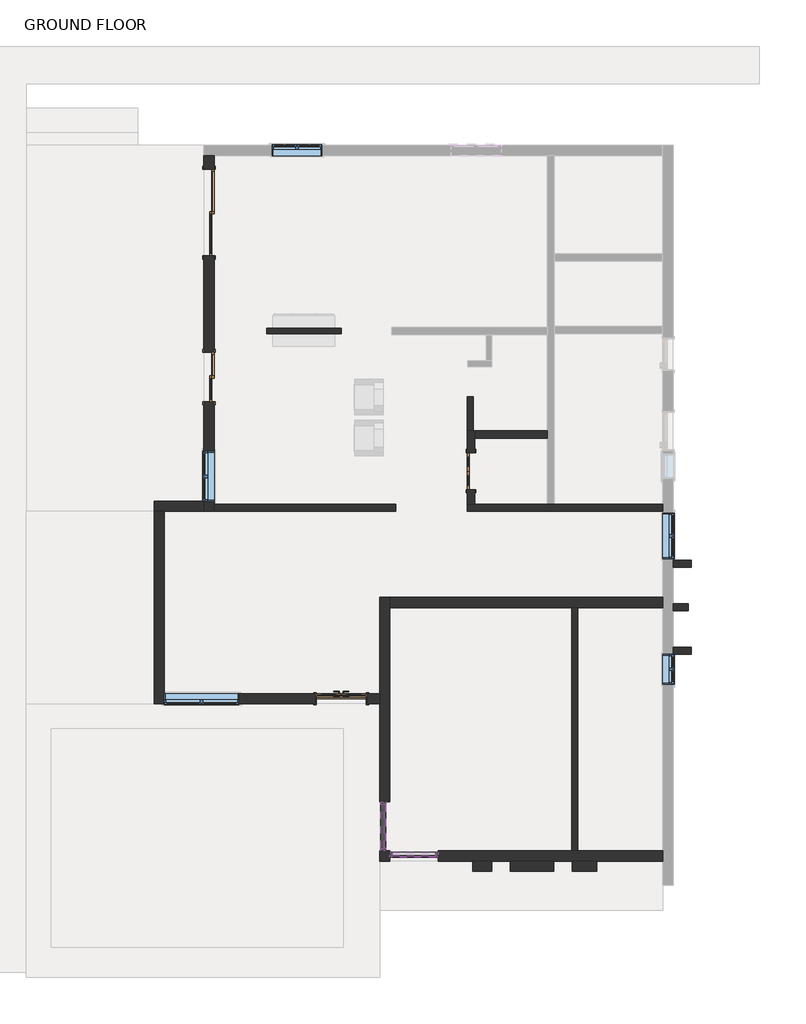
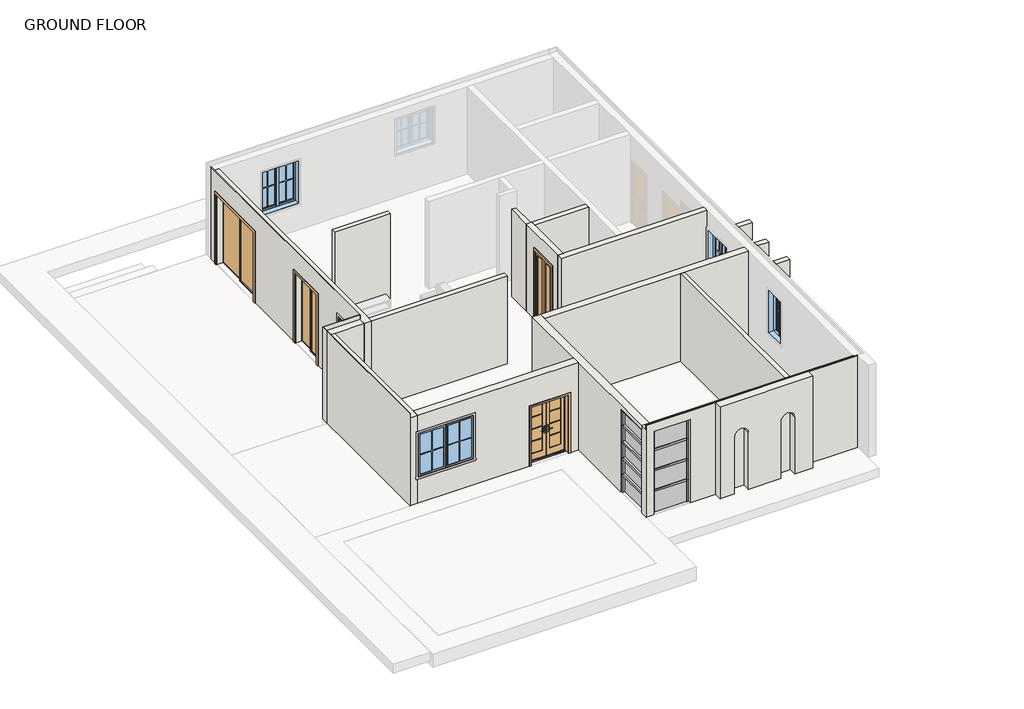
# One storey, part 1 of 2: 27 members, 18 walls, 9 plates, 5 windows, 4 doors.
"""IFC4 building model written with IfcOpenShell, lengths in millimetres."""

from ifc_helpers import new_model, si_unit, point, frame, frame_2d, origin, place, context, project, spatial, polyline, circle_curve, trimmed, segment, composite_curve, outline, extrude, faceted_brep, transform, mapped, element, save
from components import door_double_glass_3_725c6459, door_ed536266, door_double_sliding_6_53f3f6b1, door_ae07d0c6, member_2094b4cc, member_74e81316, member_bf0a6844, member_ab4f2237, member_d8a11517, member_bcb586ad, member_ae70dd35, member_aa870034, system_panel_glazed_a8ba4957, system_panel_glazed_1a26cfa3, system_panel_glazed_4987496d, system_panel_glazed_ecc42322, system_panel_glazed_0a58f99c, system_panel_glazed_1dd8fbf7, window_ba8015fa, window_casement_double_4_window_a93ed6b4, window_casement_double_4_9278a0c7, window_casement_double_6_75db422f

model = new_model("IFC4")

# Units and contexts
model_context = context("Model", 3, world=origin())
ifc_project = project(units=[si_unit("LENGTHUNIT", "METRE", prefix="MILLI")], contexts=[model_context])

# Site, building, storey
site = spatial("IfcSite", under=ifc_project)
building = spatial("IfcBuilding", under=site)
storey = spatial("IfcBuildingStorey", under=building, Name="GROUND FLOOR", Elevation=457.2)

# Doors
placement = place(None, origin())
door_double_glass_3_shape = door_double_glass_3_725c6459(model_context)
element("IfcDoor", 1, ObjectType="Door-Double-Glass : 3'", at=placement, inside=storey, context=model_context, shape_type="MappedRepresentation", body=[
    mapped(door_double_glass_3_shape, transform((1280.5251137, 1477.9935985, 457.2), x_axis=(0.0, 1.0, 0.0), y_axis=(-1.0, 0.0, 0.0), z_axis=(0.0, 0.0, 1.0))),
])
door_shape = door_ed536266(model_context)
element("IfcDoor", 2, ObjectType="Door-Double-Sliding : 48\" x 96\"", at=placement, inside=storey, context=model_context, shape_type="MappedRepresentation", body=[
    mapped(door_shape, transform((-5287.7561363, 3789.1221373, 457.2), x_axis=(0.0, -1.0, 0.0), y_axis=(1.0, 0.0, 0.0), z_axis=(0.0, 0.0, 1.0))),
])
door_double_sliding_6_shape = door_double_sliding_6_53f3f6b1(model_context)
element("IfcDoor", 3, ObjectType="Door-Double-Sliding : 6'", at=placement, inside=storey, context=model_context, shape_type="MappedRepresentation", body=[
    mapped(door_double_sliding_6_shape, transform((-5287.7561363, 7827.9935985, 457.2), x_axis=(0.0, -1.0, 0.0), y_axis=(1.0, 0.0, 0.0), z_axis=(0.0, 0.0, 1.0))),
])
door_2_shape = door_ae07d0c6(model_context)
element("IfcDoor", 4, ObjectType="Door-Exterior-Double-Full Glass-Wood_Clad : 48\" x 80\"", at=placement, inside=storey, context=model_context, shape_type="MappedRepresentation", body=[
    mapped(door_2_shape, transform((-1909.5561363, -4106.9516767, 457.2), x_axis=(1.0, 0.0, 0.0), y_axis=(0.0, 1.0, 0.0), z_axis=(0.0, 0.0, 1.0))),
])

# Members
member_shape = member_2094b4cc(model_context)
element("IfcMember", 5, ObjectType="Rectangular Mullion : 2.5\" x 5\" rectangular", at=placement, inside=storey, context=model_context, shape_type="MappedRepresentation", body=[
    mapped(member_shape, transform((-652.2561363, -7945.4064015, 3352.8), x_axis=(0.0, 0.0, 1.0), y_axis=(0.0, 1.0, 0.0), z_axis=(-1.0, 0.0, 0.0))),
])
member_2_shape = member_74e81316(model_context)
element("IfcMember", 6, ObjectType="Rectangular Mullion : 2.5\" x 5\" rectangular", at=placement, inside=storey, context=model_context, shape_type="MappedRepresentation", body=[
    mapped(member_2_shape, transform((-874.5061363, -7780.3064015, 3352.8), x_axis=(0.0, 0.0, 1.0), y_axis=(-1.0, 0.0, 0.0), z_axis=(0.0, -1.0, 0.0))),
])
member_3_shape = member_bf0a6844(model_context)
element("IfcMember", 7, ObjectType="Rectangular Mullion : 2.5\" x 5\" rectangular", at=placement, inside=storey, context=model_context, shape_type="MappedRepresentation", body=[
    mapped(member_3_shape, transform((-874.5061363, -7780.3064015, 2783.84), x_axis=(0.0, 0.0, 1.0), y_axis=(-1.0, 0.0, 0.0), z_axis=(0.0, -1.0, 0.0))),
])
element("IfcMember", 8, ObjectType="Rectangular Mullion : 2.5\" x 5\" rectangular", at=placement, inside=storey, context=model_context, shape_type="MappedRepresentation", body=[
    mapped(member_3_shape, transform((-874.5061363, -7780.3064015, 2214.88), x_axis=(0.0, 0.0, 1.0), y_axis=(-1.0, 0.0, 0.0), z_axis=(0.0, -1.0, 0.0))),
])
element("IfcMember", 9, ObjectType="Rectangular Mullion : 2.5\" x 5\" rectangular", at=placement, inside=storey, context=model_context, shape_type="MappedRepresentation", body=[
    mapped(member_3_shape, transform((-874.5061363, -7780.3064015, 1645.92), x_axis=(0.0, 0.0, 1.0), y_axis=(-1.0, 0.0, 0.0), z_axis=(0.0, -1.0, 0.0))),
])
element("IfcMember", 10, ObjectType="Rectangular Mullion : 2.5\" x 5\" rectangular", at=placement, inside=storey, context=model_context, shape_type="MappedRepresentation", body=[
    mapped(member_3_shape, transform((-874.5061363, -7780.3064015, 1076.96), x_axis=(0.0, 0.0, 1.0), y_axis=(-1.0, 0.0, 0.0), z_axis=(0.0, -1.0, 0.0))),
])
member_4_shape = member_ab4f2237(model_context)
element("IfcMember", 11, ObjectType="Rectangular Mullion : 2.5\" x 5\" rectangular", at=placement, inside=storey, context=model_context, shape_type="MappedRepresentation", body=[
    mapped(member_4_shape, transform((-874.5061363, -6637.3064015, 3352.8), x_axis=(0.0, 1.0, 0.0), y_axis=(-1.0, 0.0, 0.0), z_axis=(0.0, 0.0, 1.0))),
])
element("IfcMember", 12, ObjectType="Rectangular Mullion : 2.5\" x 5\" rectangular", at=placement, inside=storey, context=model_context, shape_type="MappedRepresentation", body=[
    mapped(member_4_shape, transform((-874.5061363, -7843.8064015, 2783.84), x_axis=(0.0, -1.0, 0.0), y_axis=(-1.0, 0.0, 0.0), z_axis=(0.0, 0.0, -1.0))),
])
element("IfcMember", 13, ObjectType="Rectangular Mullion : 2.5\" x 5\" rectangular", at=placement, inside=storey, context=model_context, shape_type="MappedRepresentation", body=[
    mapped(member_4_shape, transform((-874.5061363, -6637.3064015, 2783.84), x_axis=(0.0, 1.0, 0.0), y_axis=(-1.0, 0.0, 0.0), z_axis=(0.0, 0.0, 1.0))),
])
element("IfcMember", 14, ObjectType="Rectangular Mullion : 2.5\" x 5\" rectangular", at=placement, inside=storey, context=model_context, shape_type="MappedRepresentation", body=[
    mapped(member_4_shape, transform((-874.5061363, -6637.3064015, 2214.88), x_axis=(0.0, 1.0, 0.0), y_axis=(-1.0, 0.0, 0.0), z_axis=(0.0, 0.0, 1.0))),
])
element("IfcMember", 15, ObjectType="Rectangular Mullion : 2.5\" x 5\" rectangular", at=placement, inside=storey, context=model_context, shape_type="MappedRepresentation", body=[
    mapped(member_4_shape, transform((-874.5061363, -6637.3064015, 1645.92), x_axis=(0.0, 1.0, 0.0), y_axis=(-1.0, 0.0, 0.0), z_axis=(0.0, 0.0, 1.0))),
])
element("IfcMember", 16, ObjectType="Rectangular Mullion : 2.5\" x 5\" rectangular", at=placement, inside=storey, context=model_context, shape_type="MappedRepresentation", body=[
    mapped(member_4_shape, transform((-874.5061363, -7843.8064015, 2214.88), x_axis=(0.0, -1.0, 0.0), y_axis=(-1.0, 0.0, 0.0), z_axis=(0.0, 0.0, -1.0))),
])
element("IfcMember", 17, ObjectType="Rectangular Mullion : 2.5\" x 5\" rectangular", at=placement, inside=storey, context=model_context, shape_type="MappedRepresentation", body=[
    mapped(member_4_shape, transform((-874.5061363, -7843.8064015, 1645.92), x_axis=(0.0, -1.0, 0.0), y_axis=(-1.0, 0.0, 0.0), z_axis=(0.0, 0.0, -1.0))),
])
element("IfcMember", 18, ObjectType="Rectangular Mullion : 2.5\" x 5\" rectangular", at=placement, inside=storey, context=model_context, shape_type="MappedRepresentation", body=[
    mapped(member_4_shape, transform((-874.5061363, -7843.8064015, 1076.96), x_axis=(0.0, -1.0, 0.0), y_axis=(-1.0, 0.0, 0.0), z_axis=(0.0, 0.0, -1.0))),
])
member_5_shape = member_d8a11517(model_context)
element("IfcMember", 19, ObjectType="Rectangular Mullion : 2.5\" x 5\" rectangular", at=placement, inside=storey, context=model_context, shape_type="MappedRepresentation", body=[
    mapped(member_5_shape, transform((-874.5061363, -7843.8064015, 457.2), x_axis=(0.0, -1.0, 0.0), y_axis=(-1.0, 0.0, 0.0), z_axis=(0.0, 0.0, -1.0))),
])
element("IfcMember", 20, ObjectType="Rectangular Mullion : 2.5\" x 5\" rectangular", at=placement, inside=storey, context=model_context, shape_type="MappedRepresentation", body=[
    mapped(member_5_shape, transform((-874.5061363, -6637.3064015, 1076.96), x_axis=(0.0, 1.0, 0.0), y_axis=(-1.0, 0.0, 0.0), z_axis=(0.0, 0.0, 1.0))),
])
member_6_shape = member_bcb586ad(model_context)
element("IfcMember", 21, ObjectType="Rectangular Mullion : 2.5\" x 5\" rectangular", at=placement, inside=storey, context=model_context, shape_type="MappedRepresentation", body=[
    mapped(member_6_shape, transform((-652.2561363, -7945.4064015, 2641.6), x_axis=(0.0, 0.0, 1.0), y_axis=(0.0, 1.0, 0.0), z_axis=(-1.0, 0.0, 0.0))),
])
element("IfcMember", 22, ObjectType="Rectangular Mullion : 2.5\" x 5\" rectangular", at=placement, inside=storey, context=model_context, shape_type="MappedRepresentation", body=[
    mapped(member_6_shape, transform((-652.2561363, -7945.4064015, 1930.4), x_axis=(0.0, 0.0, 1.0), y_axis=(0.0, 1.0, 0.0), z_axis=(-1.0, 0.0, 0.0))),
])
element("IfcMember", 23, ObjectType="Rectangular Mullion : 2.5\" x 5\" rectangular", at=placement, inside=storey, context=model_context, shape_type="MappedRepresentation", body=[
    mapped(member_6_shape, transform((-652.2561363, -7945.4064015, 1219.2), x_axis=(0.0, 0.0, 1.0), y_axis=(0.0, 1.0, 0.0), z_axis=(-1.0, 0.0, 0.0))),
])
member_7_shape = member_ae70dd35(model_context)
element("IfcMember", 24, ObjectType="Rectangular Mullion : 2.5\" x 5\" rectangular", at=placement, inside=storey, context=model_context, shape_type="MappedRepresentation", body=[
    mapped(member_7_shape, transform((478.3084916, -7945.4064015, 3352.8), x_axis=(1.0, 0.0, 0.0), y_axis=(0.0, 1.0, 0.0), z_axis=(0.0, 0.0, 1.0))),
])
element("IfcMember", 25, ObjectType="Rectangular Mullion : 2.5\" x 5\" rectangular", at=placement, inside=storey, context=model_context, shape_type="MappedRepresentation", body=[
    mapped(member_7_shape, transform((-715.7561363, -7945.4064015, 2641.6), x_axis=(-1.0, 0.0, 0.0), y_axis=(0.0, 1.0, 0.0), z_axis=(0.0, 0.0, -1.0))),
])
element("IfcMember", 26, ObjectType="Rectangular Mullion : 2.5\" x 5\" rectangular", at=placement, inside=storey, context=model_context, shape_type="MappedRepresentation", body=[
    mapped(member_7_shape, transform((478.3084916, -7945.4064015, 2641.6), x_axis=(1.0, 0.0, 0.0), y_axis=(0.0, 1.0, 0.0), z_axis=(0.0, 0.0, 1.0))),
])
element("IfcMember", 27, ObjectType="Rectangular Mullion : 2.5\" x 5\" rectangular", at=placement, inside=storey, context=model_context, shape_type="MappedRepresentation", body=[
    mapped(member_7_shape, transform((478.3084916, -7945.4064015, 1930.4), x_axis=(1.0, 0.0, 0.0), y_axis=(0.0, 1.0, 0.0), z_axis=(0.0, 0.0, 1.0))),
])
element("IfcMember", 28, ObjectType="Rectangular Mullion : 2.5\" x 5\" rectangular", at=placement, inside=storey, context=model_context, shape_type="MappedRepresentation", body=[
    mapped(member_7_shape, transform((-715.7561363, -7945.4064015, 1930.4), x_axis=(-1.0, 0.0, 0.0), y_axis=(0.0, 1.0, 0.0), z_axis=(0.0, 0.0, -1.0))),
])
element("IfcMember", 29, ObjectType="Rectangular Mullion : 2.5\" x 5\" rectangular", at=placement, inside=storey, context=model_context, shape_type="MappedRepresentation", body=[
    mapped(member_7_shape, transform((-715.7561363, -7945.4064015, 1219.2), x_axis=(-1.0, 0.0, 0.0), y_axis=(0.0, 1.0, 0.0), z_axis=(0.0, 0.0, -1.0))),
])
member_8_shape = member_aa870034(model_context)
element("IfcMember", 30, ObjectType="Rectangular Mullion : 2.5\" x 5\" rectangular", at=placement, inside=storey, context=model_context, shape_type="MappedRepresentation", body=[
    mapped(member_8_shape, transform((-715.7561363, -7945.4064015, 457.2), x_axis=(-1.0, 0.0, 0.0), y_axis=(0.0, 1.0, 0.0), z_axis=(0.0, 0.0, -1.0))),
])
element("IfcMember", 31, ObjectType="Rectangular Mullion : 2.5\" x 5\" rectangular", at=placement, inside=storey, context=model_context, shape_type="MappedRepresentation", body=[
    mapped(member_8_shape, transform((478.3084916, -7945.4064015, 1219.2), x_axis=(1.0, 0.0, 0.0), y_axis=(0.0, 1.0, 0.0), z_axis=(0.0, 0.0, 1.0))),
])

# Plates
system_panel_glazed_shape = system_panel_glazed_a8ba4957(model_context)
element("IfcPlate", 32, ObjectType="System Panel : Glazed", at=placement, inside=storey, context=model_context, shape_type="MappedRepresentation", body=[
    mapped(system_panel_glazed_shape, transform((-874.5061363, -7240.5564015, 2815.59), x_axis=(0.0, -1.0, 0.0), y_axis=(1.0, 0.0, 0.0), z_axis=(0.0, 0.0, 1.0))),
])
system_panel_glazed_2_shape = system_panel_glazed_1a26cfa3(model_context)
element("IfcPlate", 33, ObjectType="System Panel : Glazed", at=placement, inside=storey, context=model_context, shape_type="MappedRepresentation", body=[
    mapped(system_panel_glazed_2_shape, transform((-874.5061363, -7240.5564015, 2246.63), x_axis=(0.0, -1.0, 0.0), y_axis=(1.0, 0.0, 0.0), z_axis=(0.0, 0.0, 1.0))),
])
element("IfcPlate", 34, ObjectType="System Panel : Glazed", at=placement, inside=storey, context=model_context, shape_type="MappedRepresentation", body=[
    mapped(system_panel_glazed_2_shape, transform((-874.5061363, -7240.5564015, 1677.67), x_axis=(0.0, -1.0, 0.0), y_axis=(1.0, 0.0, 0.0), z_axis=(0.0, 0.0, 1.0))),
])
element("IfcPlate", 35, ObjectType="System Panel : Glazed", at=placement, inside=storey, context=model_context, shape_type="MappedRepresentation", body=[
    mapped(system_panel_glazed_2_shape, transform((-874.5061363, -7240.5564015, 1108.71), x_axis=(0.0, -1.0, 0.0), y_axis=(1.0, 0.0, 0.0), z_axis=(0.0, 0.0, 1.0))),
])
system_panel_glazed_3_shape = system_panel_glazed_4987496d(model_context)
element("IfcPlate", 36, ObjectType="System Panel : Glazed", at=placement, inside=storey, context=model_context, shape_type="MappedRepresentation", body=[
    mapped(system_panel_glazed_3_shape, transform((-874.5061363, -7240.5564015, 457.2), x_axis=(0.0, -1.0, 0.0), y_axis=(1.0, 0.0, 0.0), z_axis=(0.0, 0.0, 1.0))),
])
system_panel_glazed_4_shape = system_panel_glazed_ecc42322(model_context)
element("IfcPlate", 37, ObjectType="System Panel : Glazed", at=placement, inside=storey, context=model_context, shape_type="MappedRepresentation", body=[
    mapped(system_panel_glazed_4_shape, transform((-118.7238223, -7945.4064015, 2673.35), x_axis=(-1.0, 0.0, 0.0), y_axis=(0.0, -1.0, 0.0), z_axis=(0.0, 0.0, 1.0))),
])
system_panel_glazed_5_shape = system_panel_glazed_0a58f99c(model_context)
element("IfcPlate", 38, ObjectType="System Panel : Glazed", at=placement, inside=storey, context=model_context, shape_type="MappedRepresentation", body=[
    mapped(system_panel_glazed_5_shape, transform((-118.7238223, -7945.4064015, 1962.15), x_axis=(-1.0, 0.0, 0.0), y_axis=(0.0, -1.0, 0.0), z_axis=(0.0, 0.0, 1.0))),
])
element("IfcPlate", 39, ObjectType="System Panel : Glazed", at=placement, inside=storey, context=model_context, shape_type="MappedRepresentation", body=[
    mapped(system_panel_glazed_5_shape, transform((-118.7238223, -7945.4064015, 1250.95), x_axis=(-1.0, 0.0, 0.0), y_axis=(0.0, -1.0, 0.0), z_axis=(0.0, 0.0, 1.0))),
])
system_panel_glazed_6_shape = system_panel_glazed_1dd8fbf7(model_context)
element("IfcPlate", 40, ObjectType="System Panel : Glazed", at=placement, inside=storey, context=model_context, shape_type="MappedRepresentation", body=[
    mapped(system_panel_glazed_6_shape, transform((-118.7238223, -7945.4064015, 457.2), x_axis=(-1.0, 0.0, 0.0), y_axis=(0.0, -1.0, 0.0), z_axis=(0.0, 0.0, 1.0))),
])

# Walls
element("IfcWall", 41, ObjectType="4.5\"", at=placement, inside=storey, context=model_context, shape_type="SweptSolid", body=[
    extrude(outline(polyline([(3754.6438637, -7843.8064015), (3754.6438637, -1874.8064015), (3894.3438637, -1874.8064015), (3894.3438637, -7843.8064015), (3754.6438637, -7843.8064015)])), frame((0.0, 0.0, 457.2), z_axis=(0.0, 0.0, 1.0), x_axis=(1.0, 0.0, 0.0)), (0.0, 0.0, 1.0), 3048.0),
])
element("IfcWall", 42, ObjectType="4.5\"", at=placement, inside=storey, context=model_context, shape_type="SweptSolid", body=[
    extrude(outline(polyline([(1328.9438637, 3306.7935985), (1328.9438637, 2468.5935985), (1189.2438637, 2468.5935985), (1189.2438637, 3306.7935985), (1328.9438637, 3306.7935985)])), frame((0.0, 0.0, 457.2), z_axis=(0.0, 0.0, 1.0), x_axis=(1.0, 0.0, 0.0)), (0.0, 0.0, 1.0), 3048.0),
])
element("IfcWall", 43, ObjectType="4.5\"", at=placement, inside=storey, context=model_context, shape_type="SweptSolid", body=[
    extrude(outline(polyline([(-3743.6809093, 4989.3322749), (-1914.8809093, 4989.3322749), (-1914.8809093, 4849.6322749), (-3743.6809093, 4849.6322749), (-3743.6809093, 4989.3322749)])), frame((0.0, 0.0, 457.2), z_axis=(0.0, 0.0, 1.0), x_axis=(1.0, 0.0, 0.0)), (0.0, 0.0, 1.0), 3048.0),
])
element("IfcWall", 44, ObjectType="6\" WALL", at=placement, inside=storey, context=model_context, shape_type="Brep", body=[
    faceted_brep([(5990.1084916, 665.1935985, 457.2), (3322.8438637, 665.1935985, 457.2), (3145.0438637, 665.1935985, 457.2), (1367.0438637, 665.1935985, 457.2), (1189.2438637, 665.1935985, 457.2), (1189.2438637, 665.1935985, 3505.2), (5990.1084916, 665.1935985, 3505.2), (1189.2438637, 487.3935985, 457.2), (5990.1084916, 487.3935985, 457.2), (5990.1084916, 487.3935985, 3505.2), (1189.2438637, 487.3935985, 3505.2)], [[[0, 1, 2, 3, 4, 5, 6]], [[7, 8, 9, 10]], [[4, 3, 2, 1, 0, 8, 7]], [[8, 0, 6, 9]], [[4, 7, 10, 5]], [[6, 5, 10, 9]]]),
])
element("IfcWall", 45, ObjectType="6\" WALL", at=placement, inside=storey, context=model_context, shape_type="Brep", body=[
    faceted_brep([(1367.0438637, 1935.1935985, 2895.6), (1367.0438637, 1935.1935985, 457.2), (1367.0438637, 2290.7935985, 457.2), (1367.0438637, 2468.5935985, 457.2), (1367.0438637, 2468.5935985, 3505.2), (1367.0438637, 665.1935985, 3505.2), (1367.0438637, 665.1935985, 457.2), (1367.0438637, 1020.7935985, 457.2), (1367.0438637, 1020.7935985, 2895.6), (1189.2438637, 1935.1935985, 457.2), (1189.2438637, 1935.1935985, 2895.6), (1189.2438637, 1020.7935985, 2895.6), (1189.2438637, 1020.7935985, 457.2), (1189.2438637, 665.1935985, 457.2), (1189.2438637, 665.1935985, 3505.2), (1189.2438637, 2468.5935985, 3505.2), (1189.2438637, 2468.5935985, 457.2), (1328.9438637, 2468.5935985, 457.2)], [[[0, 1, 2, 3, 4, 5, 6, 7, 8]], [[9, 10, 11, 12, 13, 14, 15, 16]], [[6, 13, 12, 7]], [[16, 17, 3, 2, 1, 9]], [[13, 6, 5, 14]], [[3, 17, 16, 15, 4]], [[10, 9, 1, 0]], [[11, 10, 0, 8]], [[12, 11, 8, 7]], [[5, 4, 15, 14]]]),
])
element("IfcWall", 46, ObjectType="6\" WALL", at=placement, inside=storey, context=model_context, shape_type="SweptSolid", body=[
    extrude(outline(polyline([(3145.0438637, 2290.7935985), (1367.0438637, 2290.7935985), (1367.0438637, 2468.5935985), (3145.0438637, 2468.5935985), (3145.0438637, 2290.7935985)])), frame((0.0, 0.0, 457.2), z_axis=(0.0, 0.0, 1.0), x_axis=(1.0, 0.0, 0.0)), (0.0, 0.0, 1.0), 3048.0),
])
element("IfcWall", 47, ObjectType="6\" WALL", at=placement, inside=storey, context=model_context, shape_type="SweptSolid", body=[
    extrude(outline(polyline([(-5033.7561363, 664.9221371), (-576.2004467, 664.9221371), (-576.2004467, 487.1221371), (-5033.7561363, 487.1221371), (-5033.7561363, 664.9221371)])), frame((0.0, 0.0, 457.2), z_axis=(0.0, 0.0, 1.0), x_axis=(1.0, 0.0, 0.0)), (0.0, 0.0, 1.0), 3048.0),
])
element("IfcWall", 48, ObjectType="6\" WALL", at=placement, inside=storey, context=model_context, shape_type="SweptSolid", body=[
    extrude(outline(polyline([(6688.3438637, -885.2318739), (6244.1084916, -885.2318739), (6244.1084916, -707.4318739), (6688.3438637, -707.4318739), (6688.3438637, -885.2318739)])), frame((0.0, 0.0, 457.2), z_axis=(0.0, 0.0, 1.0), x_axis=(1.0, 0.0, 0.0)), (0.0, 0.0, 1.0), 3200.4),
])
element("IfcWall", 49, ObjectType="6\" WALL", at=placement, inside=storey, context=model_context, shape_type="SweptSolid", body=[
    extrude(outline(polyline([(6244.1084916, -2840.9358398), (6688.3438637, -2840.9358398), (6688.3438637, -3018.7358398), (6244.1084916, -3018.7358398), (6244.1084916, -2840.9358398)])), frame((0.0, 0.0, 457.2), z_axis=(0.0, 0.0, 1.0), x_axis=(1.0, 0.0, 0.0)), (0.0, 0.0, 1.0), 3200.4),
])
element("IfcWall", 50, ObjectType="6\" WALL", at=placement, inside=storey, context=model_context, shape_type="SweptSolid", body=[
    extrude(outline(polyline([(6244.1084916, -1774.2318739), (6612.1438637, -1774.2318739), (6612.1438637, -1952.0318739), (6244.1084916, -1952.0318739), (6244.1084916, -1774.2318739)])), frame((0.0, 0.0, 457.2), z_axis=(0.0, 0.0, 1.0), x_axis=(1.0, 0.0, 0.0)), (0.0, 0.0, 1.0), 3200.4),
])
element("IfcWall", 51, ObjectType="9\"", at=placement, inside=storey, context=model_context, shape_type="Brep", body=[
    faceted_brep([(5990.1084916, -8097.8064015, 3657.6), (-969.7561363, -8097.8064015, 3657.6), (-969.7561363, -8097.8064015, 457.2), (-715.7561363, -8097.8064015, 457.2), (-715.7561363, -8097.8064015, 3352.8), (478.3084916, -8097.8064015, 3352.8), (478.3084916, -8097.8064015, 457.2), (5990.1084916, -8097.8064015, 457.2), (5990.1084916, -7843.8064015, 457.2), (3894.3438637, -7843.8064015, 457.2), (3754.6438637, -7843.8064015, 457.2), (478.3084916, -7843.8064015, 457.2), (478.3084916, -7843.8064015, 3352.8), (-715.7561363, -7843.8064015, 3352.8), (-715.7561363, -7843.8064015, 457.2), (-969.7561363, -7843.8064015, 457.2), (-969.7561363, -7843.8064015, 3352.8), (-969.7561363, -7843.8064015, 3505.2), (-715.7561363, -7843.8064015, 3505.2), (3754.6438637, -7843.8064015, 3505.2), (3894.3438637, -7843.8064015, 3505.2), (5990.1084916, -7843.8064015, 3505.2), (5990.1084916, -8085.1064015, 3657.6), (-969.7561363, -8085.1064015, 3657.6), (5990.1084916, -8085.1064015, 3505.2), (-969.7561363, -8085.1064015, 3505.2)], [[[0, 1, 2, 3, 4, 5, 6, 7]], [[8, 9, 10, 11, 12, 13, 14, 15, 16, 17, 18, 19, 20, 21]], [[8, 7, 6, 11, 10, 9]], [[3, 2, 15, 14]], [[1, 0, 22, 23]], [[0, 7, 8, 21, 24, 22]], [[5, 12, 11, 6]], [[12, 5, 4, 13]], [[13, 4, 3, 14]], [[2, 1, 23, 25, 17, 16, 15]], [[25, 24, 21, 20, 19, 18, 17]], [[24, 25, 23, 22]]]),
])
element("IfcWall", 52, ObjectType="9\"", at=placement, inside=storey, context=model_context, shape_type="Brep", body=[
    faceted_brep([(-5287.7561363, 9224.9935985, 3657.6), (-5287.7561363, 9224.9935985, 457.2), (-5287.7561363, 8894.7935985, 457.2), (-5287.7561363, 8894.7935985, 2895.6), (-5287.7561363, 6761.1935985, 2895.6), (-5287.7561363, 6761.1935985, 457.2), (-5287.7561363, 4398.7221373, 457.2), (-5287.7561363, 4398.7221373, 2895.6), (-5287.7561363, 3179.5221373, 2895.6), (-5287.7561363, 3179.5221373, 457.2), (-5287.7561363, 741.1221373, 457.2), (-5287.7561363, 487.1221373, 457.2), (-5287.7561363, 487.1221373, 3505.2), (-5287.7561363, 728.4221373, 3505.2), (-5287.7561363, 728.4221373, 3657.6), (-5287.7561363, 741.1221373, 3657.6), (-5287.7561363, 1960.3221373, 1371.6), (-5287.7561363, 1960.3221373, 2895.6), (-5287.7561363, 741.1221373, 2895.6), (-5287.7561363, 741.1221373, 1371.6), (-5033.7561363, 4398.7221373, 2895.6), (-5033.7561363, 4398.7221373, 457.2), (-5033.7561363, 6761.1935985, 457.2), (-5033.7561363, 6761.1935985, 2895.6), (-5033.7561363, 8894.7935985, 2895.6), (-5033.7561363, 8894.7935985, 457.2), (-5033.7561363, 9224.9935985, 457.2), (-5033.7561363, 9224.9935985, 3505.2), (-5033.7561363, 664.9221371, 3505.2), (-5033.7561363, 487.1221373, 3505.2), (-5033.7561363, 487.1221373, 457.2), (-5033.7561363, 664.9221371, 457.2), (-5033.7561363, 3179.5221373, 457.2), (-5033.7561363, 3179.5221373, 2895.6), (-5033.7561363, 1960.3221373, 2895.6), (-5033.7561363, 1960.3221373, 1371.6), (-5033.7561363, 741.1221373, 1371.6), (-5033.7561363, 741.1221373, 2895.6), (-5275.0561363, 728.4221373, 3657.6), (-5275.0561363, 9224.9935985, 3657.6), (-5275.0561363, 9224.9935985, 3505.2), (-5275.0561363, 728.4221373, 3505.2)], [[[0, 1, 2, 3, 4, 5, 6, 7, 8, 9, 10, 11, 12, 13, 14, 15], [16, 17, 18, 19]], [[20, 21, 22, 23, 24, 25, 26, 27, 28, 29, 30, 31, 32, 33], [34, 35, 36, 37]], [[1, 26, 25, 2]], [[30, 11, 10, 9, 32, 31]], [[21, 6, 5, 22]], [[0, 15, 14, 38, 39]], [[1, 0, 39, 40, 27, 26]], [[11, 30, 29, 12]], [[35, 34, 17, 16]], [[36, 35, 16, 19]], [[37, 36, 19, 18]], [[34, 37, 18, 17]], [[21, 20, 7, 6]], [[33, 32, 9, 8]], [[20, 33, 8, 7]], [[25, 24, 3, 2]], [[23, 22, 5, 4]], [[24, 23, 4, 3]], [[40, 41, 13, 12, 29, 28, 27]], [[41, 38, 14, 13]], [[38, 41, 40, 39]]]),
])
element("IfcWall", 53, ObjectType="9\"", at=placement, inside=storey, context=model_context, shape_type="Brep", body=[
    faceted_brep([(-5287.7561363, 741.1221373, 457.2), (-6507.1004467, 741.1221373, 457.2), (-6507.1004467, 741.1221373, 3657.6), (-5287.7561363, 741.1221373, 3657.6), (-5287.7561363, 741.1221373, 2895.6), (-5287.7561363, 741.1221373, 1371.6), (-6507.1004467, 487.1221373, 457.2), (-6253.1004467, 487.1221373, 457.2), (-5287.7561363, 487.1221373, 457.2), (-5287.7561363, 487.1221373, 3505.2), (-6253.1004467, 487.1221373, 3505.2), (-6494.4004467, 487.1221373, 3505.2), (-6494.4004467, 487.1221373, 3657.6), (-6507.1004467, 487.1221373, 3657.6), (-6494.4004467, 728.4221373, 3657.6), (-5287.7561363, 728.4221373, 3657.6), (-5287.7561363, 728.4221373, 3505.2), (-6494.4004467, 728.4221373, 3505.2)], [[[0, 1, 2, 3, 4, 5]], [[6, 7, 8, 9, 10, 11, 12, 13]], [[1, 0, 8, 7, 6]], [[3, 2, 13, 12, 14, 15]], [[0, 5, 4, 3, 15, 16, 9, 8]], [[2, 1, 6, 13]], [[16, 17, 11, 10, 9]], [[17, 14, 12, 11]], [[14, 17, 16, 15]]]),
])
element("IfcWall", 54, ObjectType="9\"", at=placement, inside=storey, context=model_context, shape_type="Brep", body=[
    faceted_brep([(-6507.1004467, 487.1221373, 457.2), (-6507.1004467, -4237.1266767, 457.2), (-6507.1004467, -4237.1266767, 3657.6), (-6507.1004467, 487.1221373, 3657.6), (-6253.1004467, -4237.1266767, 457.2), (-6253.1004467, -3983.1266767, 457.2), (-6253.1004467, 487.1221373, 457.2), (-6253.1004467, 487.1221373, 3505.2), (-6253.1004467, -3983.1266767, 3505.2), (-6253.1004467, -4237.1266767, 3505.2), (-6253.1004467, -4237.1266767, 2895.6), (-6253.1004467, -4237.1266767, 1371.6), (-6494.4004467, -4237.1266767, 3657.6), (-6494.4004467, 487.1221373, 3657.6), (-6494.4004467, 487.1221373, 3505.2), (-6494.4004467, -4237.1266767, 3505.2)], [[[0, 1, 2, 3]], [[4, 5, 6, 7, 8, 9, 10, 11]], [[1, 0, 6, 5, 4]], [[3, 2, 12, 13]], [[0, 3, 13, 14, 7, 6]], [[2, 1, 4, 11, 10, 9, 15, 12]], [[14, 15, 9, 8, 7]], [[15, 14, 13, 12]]]),
])
element("IfcWall", 55, ObjectType="9\"", at=placement, inside=storey, context=model_context, shape_type="SweptSolid", body=[
    extrude(outline(polyline([(1371.6, -4424.3004467), (1371.6, -6253.1004467), (457.2, -6253.1004467), (457.2, -2544.5561363), (2514.6, -2544.5561363), (2514.6, -1274.5561363), (457.2, -1274.5561363), (457.2, -969.7561363), (3505.2, -969.7561363), (3505.2, -6253.1004467), (2895.6, -6253.1004467), (2895.6, -4424.3004467), (1371.6, -4424.3004467)])), frame((0.0, -4237.1266767, 0.0), z_axis=(0.0, 1.0, 0.0), x_axis=(0.0, 0.0, 1.0)), (0.0, 0.0, 1.0), 254.0),
])
element("IfcWall", 56, ObjectType="9\"", at=placement, inside=storey, context=model_context, shape_type="Brep", body=[
    faceted_brep([(-715.7561363, -6637.3064015, 457.2), (-715.7561363, -1874.8064015, 457.2), (-715.7561363, -1620.8064015, 457.2), (-715.7561363, -1620.8064015, 3505.2), (-715.7561363, -7843.8064015, 3505.2), (-715.7561363, -7843.8064015, 3352.8), (-715.7561363, -6637.3064015, 3352.8), (-969.7561363, -1620.8064015, 457.2), (-969.7561363, -3983.1266767, 457.2), (-969.7561363, -4237.1266767, 457.2), (-969.7561363, -6637.3064015, 457.2), (-969.7561363, -6637.3064015, 3352.8), (-969.7561363, -7843.8064015, 3352.8), (-969.7561363, -7843.8064015, 3505.2), (-969.7561363, -4237.1266767, 3505.2), (-969.7561363, -3983.1266767, 3505.2), (-969.7561363, -1620.8064015, 3505.2)], [[[0, 1, 2, 3, 4, 5, 6]], [[7, 8, 9, 10, 11, 12, 13, 14, 15, 16]], [[7, 2, 1, 0, 10, 9, 8]], [[2, 7, 16, 3]], [[12, 5, 4, 13]], [[6, 11, 10, 0]], [[11, 6, 5, 12]], [[4, 3, 16, 15, 14, 13]]]),
])
element("IfcWall", 57, ObjectType="9\"", at=placement, inside=storey, context=model_context, shape_type="Brep", body=[
    faceted_brep([(-715.7561363, -1874.8064015, 457.2), (3754.6438637, -1874.8064015, 457.2), (3894.3438637, -1874.8064015, 457.2), (5990.1084916, -1874.8064015, 457.2), (5990.1084916, -1874.8064015, 3505.2), (-715.7561363, -1874.8064015, 3505.2), (5990.1084916, -1620.8064015, 457.2), (-715.7561363, -1620.8064015, 457.2), (-715.7561363, -1620.8064015, 3505.2), (5990.1084916, -1620.8064015, 3505.2)], [[[0, 1, 2, 3, 4, 5]], [[6, 7, 8, 9]], [[3, 2, 1, 0, 7, 6]], [[7, 0, 5, 8]], [[3, 6, 9, 4]], [[5, 4, 9, 8]]]),
])
element("IfcWall", 58, ObjectType="9\"", at=placement, inside=storey, context=model_context, shape_type="SweptSolid", body=[
    extrude(outline(composite_curve([segment(polyline([(457.2, 1315.4507424), (457.2, 1786.1438637), (2438.4, 1786.1438637)]), True, "CONTINUOUS"), segment(trimmed(circle_curve(frame_2d((2438.4, 2014.7438637)), 228.6), [point((2438.4, 1786.1438637))], [point((2438.4, 2243.3438637))], True, "CARTESIAN"), True, "CONTINUOUS"), segment(polyline([(2438.4, 2243.3438637), (457.2, 2243.3438637), (457.2, 3310.1438637), (2438.4, 3310.1438637)]), True, "CONTINUOUS"), segment(trimmed(circle_curve(frame_2d((2438.4, 3538.7438637)), 228.6), [point((2438.4, 3310.1438637))], [point((2438.4, 3767.3438637))], True, "CARTESIAN"), True, "CONTINUOUS"), segment(polyline([(2438.4, 3767.3438637), (457.2, 3767.3438637), (457.2, 4363.4507424), (3657.6, 4363.4507424), (3657.6, 1315.4507424), (457.2, 1315.4507424)]), True, "CONTINUOUS")], self_intersect=False)), frame((0.0, -8351.8064015, 0.0), z_axis=(0.0, 1.0, 0.0), x_axis=(0.0, 0.0, 1.0)), (0.0, 0.0, 1.0), 254.0),
])

# Windows
window_shape = window_ba8015fa(model_context)
element("IfcWindow", 59, ObjectType="Window-Casement-Double : 2'5\"", at=placement, inside=storey, context=model_context, shape_type="MappedRepresentation", body=[
    mapped(window_shape, transform((6117.1084916, -3387.0358398, 457.2), x_axis=(0.0, -1.0, 0.0), y_axis=(1.0, 0.0, 0.0), z_axis=(0.0, 0.0, 1.0))),
])
window_casement_double_4_window_shape = window_casement_double_4_window_a93ed6b4(model_context)
element("IfcWindow", 60, ObjectType="Window-Casement-Double : 4 window", at=placement, inside=storey, context=model_context, shape_type="MappedRepresentation", body=[
    mapped(window_casement_double_4_window_shape, transform((-5160.7561363, 1350.7221373, 457.2), x_axis=(0.0, 1.0, 0.0), y_axis=(-1.0, 0.0, 0.0), z_axis=(0.0, 0.0, 1.0))),
])
element("IfcWindow", 61, ObjectType="Window-Casement-Double : 4 window", at=placement, inside=storey, context=model_context, shape_type="MappedRepresentation", body=[
    mapped(window_casement_double_4_window_shape, transform((-2996.5357334, 9351.9935985, 457.2), x_axis=(1.0, 0.0, 0.0), y_axis=(0.0, 1.0, 0.0), z_axis=(0.0, 0.0, 1.0))),
])
window_casement_double_4_shape = window_casement_double_4_9278a0c7(model_context)
element("IfcWindow", 62, ObjectType="Window-Casement-Double : 4'", at=placement, inside=storey, context=model_context, shape_type="MappedRepresentation", body=[
    mapped(window_casement_double_4_shape, transform((6117.1084916, -110.0191377, 457.2), x_axis=(0.0, -1.0, 0.0), y_axis=(1.0, 0.0, 0.0), z_axis=(0.0, 0.0, 1.0))),
])
window_casement_double_6_shape = window_casement_double_6_75db422f(model_context)
element("IfcWindow", 63, ObjectType="Window-Casement-Double : 6'", at=placement, inside=storey, context=model_context, shape_type="MappedRepresentation", body=[
    mapped(window_casement_double_6_shape, transform((-5338.7004467, -4110.1266767, 457.2), x_axis=(-1.0, 0.0, 0.0), y_axis=(0.0, -1.0, 0.0), z_axis=(0.0, 0.0, 1.0))),
])

save(model, "model.ifc")

# Revit data of these elements
# Type "Door-Double-Glass : 3'"
#   Type Mark = "14"
#   Construction Type Id = "opn-d45"
#   Assembly Code = "C1020"
#   Analytic Construction = "Wood frame, double glass door "
#   W = 1' - 6"
#   Thickness = 0' - 2"
#   Thermal Resistance (R) = 1.8150 (h·ft²·°F)/BTU
#   Swing Angle [instance default] = 90.00°
#   Heat Transfer Coefficient (U) = 0.5510 BTU/(h·ft²·°F)
#   Height = 8' - 0"
#   Bottom Rail = 0' - 4"
#   Top Rail = 0' - 4"
#   Stiles = 0' - 4"
#   Trim Projection = 0' - 1"
#   Trim Width = 0' - 3"
#   Width = 3' - 0"
#   Define Thermal Properties by = 1
#   Glazing = Glass
#   Panel Material = Wood - Birch - Solid Stained Light Low Gloss
#   Trim Material = Paint - Sienna
#   Visual Light Transmittance = 0
#   Solar Heat Gain Coefficient = 0
#   Function = (empty or 0)
#   Wall Closure = (empty or 0)
# Type "Door-Double-Sliding : 48\" x 96\""
#   Type Mark = "8"
#   Construction Type Id = "opn-d45"
#   Assembly Code = "C1020"
#   Analytic Construction = "Wood frame, double glass door "
#   Thickness = 0' - 2"
#   Thermal Resistance (R) = 1.8150 (h·ft²·°F)/BTU
#   Heat Transfer Coefficient (U) = 0.5510 BTU/(h·ft²·°F)
#   Height = 8' - 0"
#   Rail Width = 0' - 2"
#   Stiles = 0' - 2"
#   Trim Projection Ext = 0' - 1"
#   Trim Projection Int = 0' - 1"
#   Trim Width = 0' - 3"
#   Width = 4' - 0"
#   Define Thermal Properties by = 1
#   Glazing = Glass
#   Panel Material = Wood - Birch - Solid Stained Light Low Gloss
#   Trim Material = Paint - Sienna
#   Visual Light Transmittance = 0
#   Solar Heat Gain Coefficient = 0
#   Function = (empty or 0)
#   Wall Closure = (empty or 0)
# Type "Door-Double-Sliding : 6'"
#   Type Mark = "9"
#   Construction Type Id = "opn-d45"
#   Assembly Code = "C1020"
#   Analytic Construction = "Wood frame, double glass door "
#   Thickness = 0' - 2"
#   Thermal Resistance (R) = 1.8150 (h·ft²·°F)/BTU
#   Heat Transfer Coefficient (U) = 0.5510 BTU/(h·ft²·°F)
#   Height = 8' - 0"
#   Rail Width = 0' - 2"
#   Stiles = 0' - 2"
#   Trim Projection Ext = 0' - 1"
#   Trim Projection Int = 0' - 1"
#   Trim Width = 0' - 3"
#   Width = 7' - 0"
#   Define Thermal Properties by = 1
#   Glazing = Glass
#   Panel Material = Wood - Birch - Solid Stained Light Low Gloss
#   Trim Material = Paint - Sienna
#   Visual Light Transmittance = 0
#   Solar Heat Gain Coefficient = 0
#   Function = (empty or 0)
#   Wall Closure = (empty or 0)
# Type "Door-Exterior-Double-Full Glass-Wood_Clad : 48\" x 80\""
#   Type Mark = "16"
#   Assembly Code = "B2030100"
#   Analytic Construction = "French door, wood frame with double glass"
#   Top Rail = 0' - 4 11/16"
#   Threshold Offset [instance default] = 0' - 0 1/2"
#   Thickness = 0' - 1 3/8"
#   Thermal Resistance (R) = 1.9158 (h·ft²·°F)/BTU
#   Swing Angle [instance default] = 90.00°
#   Stiles = 0' - 4 3/4"
#   Rough Width = 4' - 2"
#   Rough Height = 6' - 9"
#   Panel Width = 2' - 0"
#   Door Offset [instance default] = 0' - 0"
#   Height = 6' - 8"
#   Width = 4' - 0"
#   Heat Transfer Coefficient (U) = 0.5220 BTU/(h·ft²·°F)
#   Bottom Rail = 0' - 9 1/8"
#   Exterior Trim [instance default] = yes
#   Threshold [instance default] = yes
#   Show Grill [instance default] = yes
#   Function = 1
#   Trim Material = Cherry
#   Threshold Material = Cherry
#   Panel Material = Cherry
#   Glazing = Glass
#   Frame Material = Cherry
#   Door Handle Material = Aluminum
#   Visual Light Transmittance = 0
#   Solar Heat Gain Coefficient = 0
#   Wall Closure = (empty or 0)
#   Construction Type = (empty or 0)
# Type "Rectangular Mullion : 2.5\" x 5\" rectangular"
#   built-in parameter 1007304 = 0.416667 (stored number, unit not read)
#   built-in parameter 1007301 = 0.104167 (stored number, unit not read)
#   built-in parameter 1007300 = 0.104167 (stored number, unit not read)
# Type "System Panel : Glazed"
#   Construction Type Id = "GSP4R"
#   Analytic Construction = "1/8 in Pilkington single glazing"
#   Visual Light Transmittance = 0.9
#   Solar Heat Gain Coefficient = 0.86
#   Heat Transfer Coefficient (U) = 1.18115 BTU/(h·ft²·°F)
#   Define Thermal Properties by = 1
# Type "4.5\""
#   Assembly Code = "B2010"
#   Layers, outside or top first: 0' - 0 1/2" no material (function 4); 0' - 4 1/2" "Acoustic Ceiling Tile 24 x 24" (function 1); 0' - 0 1/2" no material (function 4)
# Type "6\" WALL"
#   Assembly Code = "B2010"
#   Layers, outside or top first: 0' - 0 1/2" no material (function 4); 0' - 6" no material (function 1); 0' - 0 1/2" no material (function 4)
# Type "9\""
#   Assembly Code = "B2010"
#   Layers, outside or top first: 0' - 0 1/2" no material (function 4); 0' - 9" no material (function 1); 0' - 0 1/2" no material (function 4)
# Type "Window-Casement-Double : 2'5\""
#   Type Mark = "19"
#   Fire Rating = "0.5h"
#   Assembly Code = "B2020100"
#   Analytic Construction = "Double glazing - domestic"
#   Frame Extension [instance default] = 0' - 0 1/4"
#   Window Inset [instance default] = 0' - 0"
#   Wall Thickness [instance default] = 0' - 6"
#   Interior Wall Closure [instance default] = 0' - 2 1/4"
#   Half Width = 1' - 2 1/2"
#   Visual Light Transmittance = 0.81
#   Thermal Resistance (R) = 1.8146 (h·ft²·°F)/BTU
#   Solar Heat Gain Coefficient = 0.76
#   Rough Width = 2' - 5 1/2"
#   Rough Height = 5' - 0 1/2"
#   Height = 5' - 0"
#   Heat Transfer Coefficient (U) = 0.5511 BTU/(h·ft²·°F)
#   Exterior Wall Closure [instance default] = 0' - 1 1/4"
#   Extension Jamb [instance default] = 0' - 2 1/4"
#   Default Sill Height = 3' - 0"
#   Width = 2' - 5"
#   Muntin Visibility = yes
#   Interior Trim Visibility [instance default] = yes
#   Exterior Trim Visibility [instance default] = yes
#   Extension Jamb Visibility [instance default] = yes
#   Interior Trim Material = Wood - Stained
#   Muntin Pattern = Muntin Pattern_2x2 : Muntin Pattern_2x2
#   Interior Trim = Trim-Window-Interior-Flat : Picture Frame
#   Interior Frame Material = Wood - Stained
#   Glass Panel Material = Glass
#   Exterior Trim Material = Clad - White
#   Exterior Trim = Trim-Window-Exterior-Flat : with Sill
#   Exterior Frame Material = Clad - White
#   Wall Closure = (empty or 0)
# Type "Window-Casement-Double : 4 window"
#   Type Mark = "21"
#   Fire Rating = "0.5h"
#   Assembly Code = "B2020100"
#   Analytic Construction = "Double glazing - domestic"
#   Frame Extension [instance default] = 0' - 0 1/4"
#   Window Inset [instance default] = 0' - 0"
#   Wall Thickness [instance default] = 0' - 6"
#   Interior Wall Closure [instance default] = 0' - 2 1/4"
#   Half Width = 2' - 0"
#   Visual Light Transmittance = 0.81
#   Thermal Resistance (R) = 1.8146 (h·ft²·°F)/BTU
#   Solar Heat Gain Coefficient = 0.76
#   Rough Width = 4' - 0 1/2"
#   Rough Height = 5' - 0 1/2"
#   Height = 5' - 0"
#   Heat Transfer Coefficient (U) = 0.5511 BTU/(h·ft²·°F)
#   Exterior Wall Closure [instance default] = 0' - 1 1/4"
#   Extension Jamb [instance default] = 0' - 2 1/4"
#   Default Sill Height = 3' - 0"
#   Width = 4' - 0"
#   Muntin Visibility = yes
#   Interior Trim Visibility [instance default] = yes
#   Exterior Trim Visibility [instance default] = yes
#   Extension Jamb Visibility [instance default] = yes
#   Interior Trim Material = Wood - Stained
#   Muntin Pattern = Muntin Pattern_2x2 : Muntin Pattern_2x2
#   Interior Trim = Trim-Window-Interior-Flat : Picture Frame
#   Interior Frame Material = Wood - Stained
#   Glass Panel Material = Glass
#   Exterior Trim Material = Clad - White
#   Exterior Trim = Trim-Window-Exterior-Flat : with Sill
#   Exterior Frame Material = Clad - White
#   Wall Closure = (empty or 0)
# Type "Window-Casement-Double : 4'"
#   Type Mark = "18"
#   Fire Rating = "0.5h"
#   Assembly Code = "B2020100"
#   Analytic Construction = "Double glazing - domestic"
#   Frame Extension [instance default] = 0' - 0 1/4"
#   Window Inset [instance default] = 0' - 0"
#   Wall Thickness [instance default] = 0' - 6"
#   Interior Wall Closure [instance default] = 0' - 2 1/4"
#   Half Width = 1' - 10"
#   Visual Light Transmittance = 0.81
#   Thermal Resistance (R) = 1.8146 (h·ft²·°F)/BTU
#   Solar Heat Gain Coefficient = 0.76
#   Rough Width = 3' - 8 1/2"
#   Rough Height = 5' - 0 1/2"
#   Height = 5' - 0"
#   Heat Transfer Coefficient (U) = 0.5511 BTU/(h·ft²·°F)
#   Exterior Wall Closure [instance default] = 0' - 1 1/4"
#   Extension Jamb [instance default] = 0' - 2 1/4"
#   Default Sill Height = 3' - 0"
#   Width = 3' - 8"
#   Muntin Visibility = yes
#   Interior Trim Visibility [instance default] = yes
#   Exterior Trim Visibility [instance default] = yes
#   Extension Jamb Visibility [instance default] = yes
#   Interior Trim Material = Wood - Stained
#   Muntin Pattern = Muntin Pattern_2x2 : Muntin Pattern_2x2
#   Interior Trim = Trim-Window-Interior-Flat : Picture Frame
#   Interior Frame Material = Wood - Stained
#   Glass Panel Material = Glass
#   Exterior Trim Material = Clad - White
#   Exterior Trim = Trim-Window-Exterior-Flat : with Sill
#   Exterior Frame Material = Clad - White
#   Wall Closure = (empty or 0)
# Type "Window-Casement-Double : 6'"
#   Type Mark = "20"
#   Fire Rating = "0.5h"
#   Assembly Code = "B2020100"
#   Analytic Construction = "Double glazing - domestic"
#   Frame Extension [instance default] = 0' - 0 1/4"
#   Window Inset [instance default] = 0' - 0"
#   Wall Thickness [instance default] = 0' - 6"
#   Interior Wall Closure [instance default] = 0' - 2 1/4"
#   Half Width = 3' - 0"
#   Visual Light Transmittance = 0.81
#   Thermal Resistance (R) = 1.8146 (h·ft²·°F)/BTU
#   Solar Heat Gain Coefficient = 0.76
#   Rough Width = 6' - 0 1/2"
#   Rough Height = 5' - 0 1/2"
#   Height = 5' - 0"
#   Heat Transfer Coefficient (U) = 0.5511 BTU/(h·ft²·°F)
#   Exterior Wall Closure [instance default] = 0' - 1 1/4"
#   Extension Jamb [instance default] = 0' - 2 1/4"
#   Default Sill Height = 3' - 0"
#   Width = 6' - 0"
#   Muntin Visibility = yes
#   Interior Trim Visibility [instance default] = yes
#   Exterior Trim Visibility [instance default] = yes
#   Extension Jamb Visibility [instance default] = yes
#   Interior Trim Material = Wood - Stained
#   Muntin Pattern = Muntin Pattern_2x2 : Muntin Pattern_2x2
#   Interior Trim = Trim-Window-Interior-Flat : Picture Frame
#   Interior Frame Material = Wood - Stained
#   Glass Panel Material = Glass
#   Exterior Trim Material = Clad - White
#   Exterior Trim = Trim-Window-Exterior-Flat : with Sill
#   Exterior Frame Material = Clad - White
#   Wall Closure = (empty or 0)
# Element 1 (IfcDoor, "Door-Double-Glass : 3'")
#   Swing Angle = 90.00°
#   Phase Created = New Construction
#   Materials on its faces: "Wood - Birch - Solid Stained Light Low Gloss", "Paint - Sienna", "Glass"
# Element 2 (IfcDoor, "Door-Double-Sliding : 48\" x 96\"")
#   Phase Created = New Construction
#   Materials on its faces: "Paint - Sienna", "Wood - Birch - Solid Stained Light Low Gloss", "Glass"
# Element 3 (IfcDoor, "Door-Double-Sliding : 6'")
#   Phase Created = New Construction
#   Materials on its faces: "Paint - Sienna", "Wood - Birch - Solid Stained Light Low Gloss", "Glass"
# Element 4 (IfcDoor, "Door-Exterior-Double-Full Glass-Wood_Clad : 48\" x 80\"")
#   Threshold Offset = 0' - 0 1/2"
#   Swing Angle = 90.00°
#   Door Offset = 0' - 0"
#   Threshold = yes
#   Show Grill = yes
#   Exterior Trim = yes
#   Phase Created = New Construction
#   Materials on its faces: "Cherry", "Aluminum", "Glass"
# Elements 5, 6, 7, 8, 9, 10, 11, 12, 13, 14, 15, 16, 17, 18, 19, 20, 21, 22, 23, 24, 25, 26, 27, 28, 29, 30, 31 (IfcMember, "Rectangular Mullion : 2.5\" x 5\" rectangular")
#   Phase Created = New Construction
#   Materials on its faces: "Aluminum"
# Elements 32, 33, 34, 35, 36, 37, 38, 39, 40 (IfcPlate, "System Panel : Glazed")
#   Phase Created = New Construction
#   Materials on its faces: "Glass"
# Elements 41, 42, 43 (IfcWall, "4.5\"")
#   Top Offset = 0' - 0"
#   Base Offset = 0' - 0"
#   wall height = 10' - 6"
#   Phase Created = New Construction
#   Base Constraint = GROUND FLOOR
#   Materials on its faces: "Default Wall"
# Elements 44, 45, 46, 47, 48, 49, 50 (IfcWall, "6\" WALL")
#   Top Offset = 0' - 0"
#   Base Offset = 0' - 0"
#   wall height = 10' - 6"
#   Phase Created = New Construction
#   Base Constraint = GROUND FLOOR
#   Materials on its faces: "Default Wall"
# Elements 51, 52, 53, 54, 55, 56, 57, 58 (IfcWall, "9\"")
#   Top Offset = 0' - 0"
#   Base Offset = 0' - 0"
#   wall height = 10' - 6"
#   Phase Created = New Construction
#   Base Constraint = GROUND FLOOR
#   Materials on its faces: "Default Wall"
# Element 59 (IfcWindow, "Window-Casement-Double : 2'5\"")
#   Mark = "2"
#   Window Inset = 0' - 0"
#   Interior Wall Closure = 0' - 2 1/4"
#   Frame Extension = 0' - 0 1/4"
#   Exterior Wall Closure = 0' - 1 1/4"
#   Interior Trim Visibility = yes
#   Exterior Trim Visibility = yes
#   Phase Created = New Construction
#   Materials on its faces: "Wood - Stained", "Glass", "Clad - White"
# Element 60 (IfcWindow, "Window-Casement-Double : 4 window")
#   Mark = "4"
#   Window Inset = 0' - 0"
#   Interior Wall Closure = 0' - 2 1/4"
#   Frame Extension = 0' - 0 1/4"
#   Exterior Wall Closure = 0' - 1 1/4"
#   Interior Trim Visibility = yes
#   Exterior Trim Visibility = yes
#   Phase Created = New Construction
#   Materials on its faces: "Wood - Stained", "Glass", "Clad - White"
# Element 61 (IfcWindow, "Window-Casement-Double : 4 window")
#   Mark = "5"
#   Window Inset = 0' - 0"
#   Interior Wall Closure = 0' - 2 1/4"
#   Frame Extension = 0' - 0 1/4"
#   Exterior Wall Closure = 0' - 1 1/4"
#   Interior Trim Visibility = yes
#   Exterior Trim Visibility = yes
#   Phase Created = New Construction
#   Materials on its faces: "Wood - Stained", "Glass", "Clad - White"
# Element 62 (IfcWindow, "Window-Casement-Double : 4'")
#   Mark = "1"
#   Window Inset = 0' - 0"
#   Interior Wall Closure = 0' - 2 1/4"
#   Frame Extension = 0' - 0 1/4"
#   Exterior Wall Closure = 0' - 1 1/4"
#   Interior Trim Visibility = yes
#   Exterior Trim Visibility = yes
#   Phase Created = New Construction
#   Materials on its faces: "Wood - Stained", "Glass", "Clad - White"
# Element 63 (IfcWindow, "Window-Casement-Double : 6'")
#   Mark = "3"
#   Window Inset = 0' - 0"
#   Interior Wall Closure = 0' - 2 1/4"
#   Frame Extension = 0' - 0 1/4"
#   Exterior Wall Closure = 0' - 1 1/4"
#   Interior Trim Visibility = yes
#   Exterior Trim Visibility = yes
#   Phase Created = New Construction
#   Materials on its faces: "Wood - Stained", "Glass", "Clad - White"
# Materials
#   "Glass": class "Glass", colour RGB 0 128 192, transparency 0.75, Description = "Soda Lime Glass", Cost = 0
#   "Wood - Birch - Solid Stained Light Low Gloss": class "Wood", colour RGB 210 159 95, transparency 0, Cost = 0
#   "Paint - Sienna": colour RGB 118 70 51, transparency 0, Cost = 0
#   "Cherry": class "Wood", colour RGB 226 177 128, transparency 0, Description = "Prunus Serotina", Cost = 0
#   "Aluminum": class "Metal", colour RGB 247 247 247, transparency 0, Description = "Aluminum 6061", Cost = 0
#   "Acoustic Ceiling Tile 24 x 24": class "Generic", colour RGB 232 232 232, transparency 0, Description = "Acoustic Ceiling Tile 24 x 24", Cost = 0
#   "Wood - Stained": class "Wood", colour RGB 224 178 126, transparency 0, Cost = 0
#   "Clad - White": class "Wood", colour RGB 242 242 238, transparency 0, Cost = 0
#   "Default Wall": colour RGB 128 128 128, transparency 0, Cost = 0
